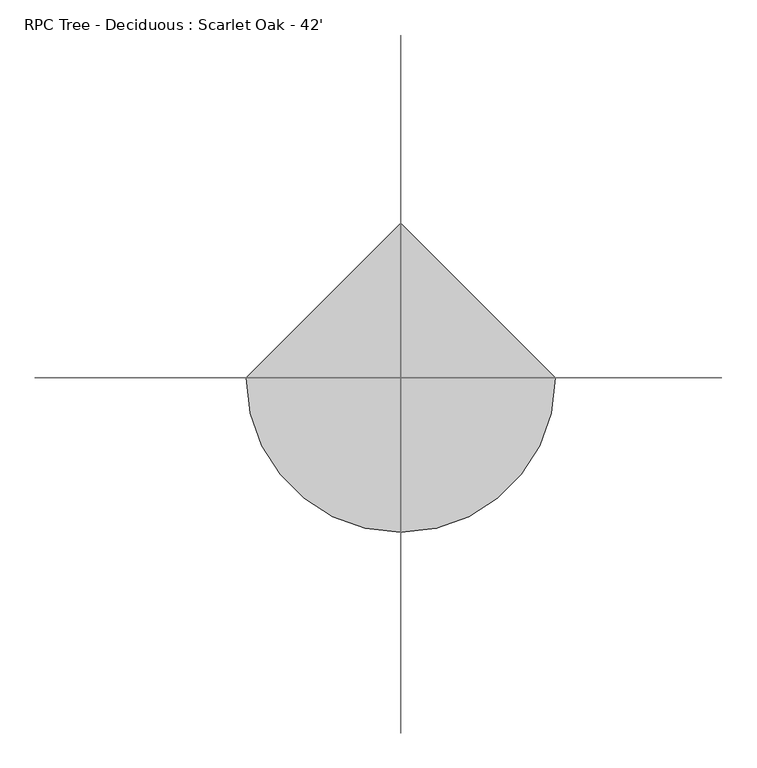
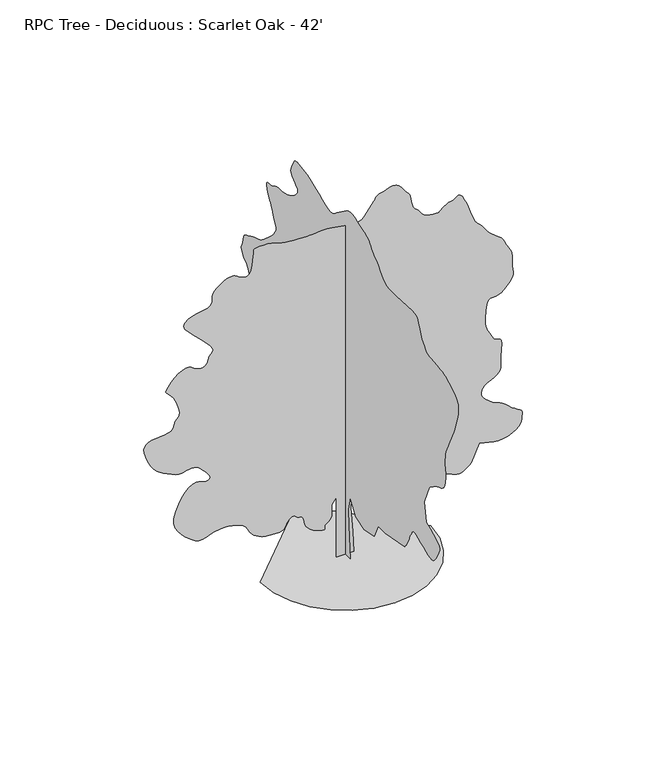
"""IFC4 building model written with IfcOpenShell, lengths in millimetres: geographic element geometry, RPC Tree - Deciduous : Scarlet Oak - 42'."""

from ifc_helpers import new_model, si_unit, origin, place, context, project, spatial, triangles, source, transform, mapped, element, save


def rpc_tree_deciduous_scarlet_oak_42_9b182cbb(model_context):
    return source(origin(), model_context, "Body", "Tessellation", [
        triangles([(0.0176667, 313.3908637, 0.0), (0.0176667, -300.6481277, 0.0), (0.0176667, -201.6098415, 1168.65294), (0.0176667, -181.8016574, 1723.2669067), (0.0176667, -300.6481277, 2238.2675938), (0.0176667, -617.5722605, 1723.2669067), (0.0176667, -1132.5703314, 1564.8060848), (0.0176667, -1726.8001213, 1703.4602669), (0.0176667, -1964.4925896, 2198.6516979), (0.0176667, -2380.4549904, 2198.6516979), (0.0176667, -3529.2988197, 2416.5375263), (0.0176667, -3571.5694954, 2467.5287453), (0.0176667, -3612.8163963, 2518.865728), (0.0176667, -3651.9637161, 2570.8942383), (0.0176667, -3687.9873894, 2623.969487), (0.0176667, -3719.8633507, 2678.4275002), (0.0176667, -3746.5419548, 2734.6266861), (0.0176667, -3766.9988457, 2792.8740028), (0.0176667, -3786.866819, 2852.8877815), (0.0176667, -3811.9324402, 2913.9259163), (0.0176667, -3841.3248322, 2975.8343468), (0.0176667, -3874.1736992, 3038.4340141), (0.0176667, -3909.6343254, 3101.5461502), (0.0176667, -3946.8099632, 3165.016404), (0.0176667, -3984.882058, 3228.6404274), (0.0176667, -4003.0091492, 3249.1996376), (0.0176667, -4028.0747704, 3265.7904854), (0.0176667, -4066.991581, 3274.393158), (0.0176667, -4126.698111, 3271.0392929), (0.0176667, -4214.133181, 3251.7599464), (0.0176667, -4336.2091599, 3212.5358871), (0.0176667, -4499.8648682, 3149.4240417), (0.0176667, -4672.6607162, 3075.1492149), (0.0176667, -4819.8023163, 3008.8625633), (0.0176667, -4944.7714325, 2956.0686928), (0.0176667, -5051.0248306, 2922.3492393), (0.0176667, -5142.0442749, 2913.2343887), (0.0176667, -5221.2603699, 2934.2546173), (0.0176667, -5292.1816223, 2990.9656906), (0.0176667, -5363.7423706, 3080.2954124), (0.0176667, -5437.7099487, 3189.0320892), (0.0176667, -5506.8388687, 3307.4725342), (0.0176667, -5563.8313202, 3425.9129791), (0.0176667, -5601.4168167, 3534.6496559), (0.0176667, -5612.3492889, 3624.0049576), (0.0176667, -5589.3065094, 3684.2236656), (0.0176667, -5533.0052948, 3729.5668282), (0.0176667, -5451.7404877, 3780.0820587), (0.0176667, -5349.7118317, 3834.9496399), (0.0176667, -5231.0155884, 3893.2736961), (0.0176667, -5099.8759186, 3954.2095116), (0.0176667, -4960.4152451, 4016.8603386), (0.0176667, -4816.8068596, 4080.3820427), (0.0176667, -4697.9568466, 4753.8484932), (0.0176667, -4995.0561539, 5447.1064682), (0.0176667, -5004.4270935, 5460.3434509), (0.0176667, -5018.9698105, 5476.4988602), (0.0176667, -5043.9328217, 5498.5690247), (0.0176667, -5084.4629059, 5529.4717896), (0.0176667, -5145.7824188, 5572.1267441), (0.0176667, -5233.1148788, 5629.5290543), (0.0176667, -5351.6064835, 5704.6233078), (0.0176667, -5480.1602646, 5772.6511322), (0.0176667, -5594.1457489, 5817.0984192), (0.0176667, -5693.5885162, 5853.2497009), (0.0176667, -5778.4885666, 5896.340094), (0.0176667, -5848.8209015, 5961.6029709), (0.0176667, -5904.609938, 6064.2717041), (0.0176667, -5945.8312592, 6219.6064087), (0.0176667, -5969.6931747, 6372.1755844), (0.0176667, -5976.5549652, 6470.0056595), (0.0176667, -5971.3064484, 6533.5267822), (0.0176667, -5958.7607025, 6583.1970062), (0.0176667, -5943.8087082, 6639.4476425), (0.0176667, -5931.2885422, 6722.7088394), (0.0176667, -5926.0400253, 6853.4648117), (0.0176667, -5927.8835175, 6997.7129837), (0.0176667, -5935.9737213, 7117.3568436), (0.0176667, -5954.1011032, 7226.6309875), (0.0176667, -5986.0793839, 7339.6950165), (0.0176667, -6035.7496078, 7470.7835266), (0.0176667, -6106.9010788, 7634.1061157), (0.0176667, -6203.3225189, 7843.8473831), (0.0176667, -6294.8797211, 8033.439299), (0.0176667, -6355.9178558, 8147.834642), (0.0176667, -6397.1897552, 8218.5762543), (0.0176667, -6429.4755753, 8277.1819794), (0.0176667, -6463.5019867, 8355.1946594), (0.0176667, -6509.9718246, 8484.1577179), (0.0176667, -6579.6896622, 8695.5634186), (0.0176667, -6654.8094955, 8940.125235), (0.0176667, -6705.3500153, 9150.7373795), (0.0176667, -6723.656456, 9332.2385101), (0.0176667, -6702.0984695, 9489.4934464), (0.0176667, -6633.0980301, 9627.3408463), (0.0176667, -6508.9992096, 9750.6205307), (0.0176667, -6322.1728226, 9864.2211548), (0.0176667, -6140.9019104, 9957.5968506), (0.0176667, -6021.6679092, 10021.8859497), (0.0176667, -5939.1485275, 10064.3101044), (0.0176667, -5868.0487976, 10092.2177032), (0.0176667, -5783.0970062, 10112.8292358), (0.0176667, -5658.9987671, 10133.4396057), (0.0176667, -5470.4567871, 10161.3472046), (0.0176667, -5268.216806, 10183.3400482), (0.0176667, -5111.3717285, 10191.8406921), (0.0176667, -4987.0938492, 10202.3888855), (0.0176667, -4882.5816238, 10230.6290222), (0.0176667, -4784.982058, 10292.127594), (0.0176667, -4681.493898, 10402.5034149), (0.0176667, -4559.2897293, 10577.2962341), (0.0176667, -4452.5756035, 10769.4740387), (0.0176667, -4389.5149178, 10923.9122864), (0.0176667, -4348.2938873, 11044.0165833), (0.0176667, -4307.0469864, 11133.2960175), (0.0176667, -4243.9863007, 11195.2038666), (0.0176667, -4137.2721748, 11233.1992218), (0.0176667, -3965.0652443, 11250.763266), (0.0176667, -3014.2904297, 11191.3378235), (0.0176667, -2839.0363014, 11194.4108917), (0.0176667, -2696.349662, 11194.0004517), (0.0176667, -2575.1186897, 11201.2209412), (0.0176667, -2464.3027794, 11227.1309875), (0.0176667, -2352.7906906, 11282.8694458), (0.0176667, -2229.4985069, 11379.4705261), (0.0176667, -2083.3375156, 11528.0707581), (0.0176667, -1942.4917522, 11678.1569458), (0.0176667, -1836.9835121, 11780.4158203), (0.0176667, -1758.5045815, 11847.7012482), (0.0176667, -1698.7339565, 11892.8147736), (0.0176667, -1649.3606621, 11928.556778), (0.0176667, -1602.0639851, 11967.7555481), (0.0176667, -1548.5328049, 12023.2626251), (0.0176667, -1497.1368141, 12088.8074615), (0.0176667, -1455.0938862, 12149.8444336), (0.0176667, -1412.3621922, 12206.7351471), (0.0176667, -1358.8872585, 12259.7853973), (0.0176667, -1284.6226055, 12309.4044617), (0.0176667, -1179.5189192, 12355.8992981), (0.0176667, -1033.5320452, 12399.6036072), (0.0176667, -869.6434296, 12447.7634583), (0.0176667, -716.8409832, 12501.1206665), (0.0176667, -574.0851983, 12550.3304535), (0.0176667, -440.341763, 12586.0212982), (0.0176667, -314.5660463, 12598.8484222), (0.0176667, -195.7190492, 12579.4414673), (0.0176667, -82.7633712, 12518.4544922), (0.0176667, 511.4674361, 12082.6880676), (0.0176667, 575.7980298, 12024.1335022), (0.0176667, 638.0522604, 11970.7762939), (0.0176667, 705.8469595, 11927.7882202), (0.0176667, 786.8119303, 11900.4189606), (0.0176667, 888.5641497, 11893.8379669), (0.0176667, 1018.7282976, 11913.2460846), (0.0176667, 1184.9289087, 11963.8371826), (0.0176667, 1373.534911, 12038.957016), (0.0176667, 1563.5259304, 12123.4483704), (0.0176667, 1751.4381523, 12209.6791534), (0.0176667, 1933.8071079, 12289.996344), (0.0176667, 2107.1689098, 12356.8213348), (0.0176667, 2268.0542931, 12402.4976166), (0.0176667, 2413.0043118, 12419.4210022), (0.0176667, 2544.8429214, 12428.6634613), (0.0176667, 2667.3156784, 12449.6842712), (0.0176667, 2778.3824455, 12472.4200928), (0.0176667, 2875.9049812, 12486.8599091), (0.0176667, 2957.8610252, 12482.9427063), (0.0176667, 3022.1248352, 12450.606308), (0.0176667, 3066.6488617, 12379.7873749), (0.0176667, 3106.4362587, 12290.8160614), (0.0176667, 3152.1122498, 12208.7582794), (0.0176667, 3195.0232933, 12130.8479187), (0.0176667, 3226.5152664, 12054.318869), (0.0176667, 3237.8831772, 11976.4340881), (0.0176667, 3220.4984825, 11894.3763062), (0.0176667, 3165.7076408, 11805.3794128), (0.0176667, 3081.8572357, 11723.8332275), (0.0176667, 2992.092366, 11659.9534058), (0.0176667, 2909.982843, 11604.7532867), (0.0176667, 2848.9961586, 11549.1938873), (0.0176667, 2822.6759628, 11484.2897095), (0.0176667, 2844.4900383, 11401.0285126), (0.0176667, 2928.0076149, 11290.3713135), (0.0176667, 3043.3244133, 11180.1233917), (0.0176667, 3152.0610901, 11099.7038818), (0.0176667, 3254.9091728, 11042.4550507), (0.0176667, 3352.5598984, 11001.8738068), (0.0176667, 3445.704213, 10971.3035797), (0.0176667, 3535.0595146, 10944.2412781), (0.0176667, 3621.2652992, 10914.0291687), (0.0176667, 3707.3690552, 10890.7561707), (0.0176667, 3795.9049301, 10883.0752441), (0.0176667, 3886.8473442, 10882.333429), (0.0176667, 3980.222168, 10879.8498596), (0.0176667, 4076.0294014, 10866.9715759), (0.0176667, 4174.2690445, 10835.0177124), (0.0176667, 4274.9152267, 10775.3887939), (0.0176667, 4378.9408539, 10722.4152832), (0.0176667, 4481.2000191, 10703.4176056), (0.0176667, 4572.7316414, 10698.9632263), (0.0176667, 4644.5228989, 10689.6684448), (0.0176667, 4687.5362617, 10656.1286316), (0.0176667, 4692.7850693, 10578.9089264), (0.0176667, 4651.2820793, 10438.6546967), (0.0176667, 4589.9369865, 10291.0520782), (0.0176667, 4539.012188, 10191.6093109), (0.0176667, 4494.308812, 10120.561322), (0.0176667, 4451.7053078, 10058.1918732), (0.0176667, 4407.0019318, 9984.7358917), (0.0176667, 4356.0515533, 9880.4538849), (0.0176667, 4294.7320404, 9725.5801987), (0.0176667, 4229.9301819, 9573.2412415), (0.0176667, 4174.1664345, 9477.02444), (0.0176667, 4131.5370598, 9417.880957), (0.0176667, 4106.2412201, 9376.7625366), (0.0176667, 4102.4263367, 9334.6197601), (0.0176667, 4124.265992, 9272.3526306), (0.0176667, 4175.8820274, 9170.9640518), (0.0176667, 4267.7717674, 9036.5728363), (0.0176667, 4396.7095367, 8893.8861969), (0.0176667, 4546.4626053, 8751.5320953), (0.0176667, 4700.6962143, 8618.1908157), (0.0176667, 4843.178215, 8502.5153183), (0.0176667, 4957.5729767, 8413.1858871), (0.0176667, 5027.6233521, 8358.830484), (0.0176667, 5089.8137421, 8324.829071), (0.0176667, 5183.1888565, 8290.4695404), (0.0176667, 5295.279689, 8255.4187729), (0.0176667, 5413.6172333, 8219.3186508), (0.0176667, 5525.7080658, 8181.8354736), (0.0176667, 5619.0831802, 8142.6367035), (0.0176667, 5681.2729889, 8101.3392242), (0.0176667, 5733.3500427, 8067.0308533), (0.0176667, 5799.6622742, 8042.7846588), (0.0176667, 5872.5293381, 8019.2297012), (0.0176667, 5944.3714645, 7986.9950409), (0.0176667, 6007.5606308, 7936.7614792), (0.0176667, 6054.4397461, 7859.1324966), (0.0176667, 6077.431366, 7744.7888947), (0.0176667, 6096.2499847, 7629.9325333), (0.0176667, 6128.5869644, 7548.6938873), (0.0176667, 6163.6888916, 7488.5777893), (0.0176667, 6190.8535126, 7437.1152328), (0.0176667, 6199.277417, 7381.8633728), (0.0176667, 6178.2571884, 7310.3026245), (0.0176667, 6117.0399948, 7209.9889801), (0.0176667, 6041.0492844, 7116.0255295), (0.0176667, 5979.6018723, 7059.8522141), (0.0176667, 5927.8579376, 7023.4183914), (0.0176667, 5880.9526611, 6988.7007431), (0.0176667, 5834.0729645, 6937.699205), (0.0176667, 5782.3290298, 6852.4148758), (0.0176667, 5720.8816177, 6714.7976944), (0.0176667, 5653.9037292, 6576.9502945), (0.0176667, 5592.4557358, 6490.0526917), (0.0176667, 5542.0942749, 6434.6729324), (0.0176667, 5508.3748215, 6391.4034805), (0.0176667, 5496.8278519, 6340.8885406), (0.0176667, 5512.9832611, 6263.6694168), (0.0176667, 5562.4232666, 6140.3897324), (0.0176667, 5628.0954208, 6005.5380798), (0.0176667, 5689.9271118, 5900.8462143), (0.0176667, 5749.0194351, 5817.6361771), (0.0176667, 5806.3450058, 5747.2271027), (0.0176667, 5863.0049194, 5680.9916107), (0.0176667, 5919.9973709, 5610.2499985), (0.0176667, 5978.3728775, 5526.348143), (0.0176667, 6046.1187424, 5443.5985428), (0.0176667, 6124.9511398, 5376.0828964), (0.0176667, 6206.5484848, 5314.8145432), (0.0176667, 6282.6153534, 5250.7556625), (0.0176667, 6344.8057434, 5174.9445923), (0.0176667, 6384.8236496, 5078.3179321), (0.0176667, 6394.3480682, 4951.9151825), (0.0176667, 6402.3615326, 4852.6511833), (0.0176667, 6431.8824051, 4819.9049263), (0.0176667, 6465.5506989, 4818.343103), (0.0176667, 6486.0587494, 4812.6335678), (0.0176667, 6476.0477325, 4767.4183044), (0.0176667, 6418.2611435, 4647.3648766), (0.0176667, 6295.3145782, 4417.1152679), (0.0176667, 6166.7613785, 4158.8557411), (0.0176667, 6089.1579758, 3968.8801277), (0.0176667, 6040.640007, 3832.9270889), (0.0176667, 5999.4186859, 3736.8381866), (0.0176667, 5943.629068, 3666.3782433), (0.0176667, 5851.4579498, 3607.3629501), (0.0176667, 5701.0903839, 3545.5824188), (0.0176667, 5527.4748184, 3495.4511765), (0.0176667, 5374.6748428, 3474.4309479), (0.0176667, 5234.3438736, 3472.8179649), (0.0176667, 5098.1859055, 3480.9087502), (0.0176667, 4957.8549362, 3488.9736649), (0.0176667, 4805.0549606, 3487.3606819), (0.0176667, 4631.4652657, 3466.3404533), (0.0176667, 4458.3362984, 3447.5221252), (0.0176667, 4308.7625793, 3451.5675179), (0.0176667, 4177.2133415, 3467.3900986), (0.0176667, 4058.1328194, 3483.9042068), (0.0176667, 3945.9908272, 3490.0233101), (0.0176667, 3835.2313087, 3474.6614571), (0.0176667, 3720.2984985, 3426.7324059), (0.0176667, 3610.3072472, 3375.7820274), (0.0176667, 3519.3389626, 3349.1034233), (0.0176667, 3449.5190964, 3332.1285873), (0.0176667, 3402.9213593, 3310.3145119), (0.0176667, 3381.6194618, 3269.0679016), (0.0176667, 3387.6874054, 3193.8969086), (0.0176667, 3423.1991913, 3070.1820763), (0.0176667, 3480.4733116, 2938.7610283), (0.0176667, 3549.1923729, 2845.7701927), (0.0176667, 3627.4614326, 2784.8599571), (0.0176667, 3713.3343887, 2749.5789711), (0.0176667, 3804.9171707, 2733.5255905), (0.0176667, 3900.3145454, 2730.2740448), (0.0176667, 3997.6068626, 2733.448851), (0.0176667, 4373.9740059, 2317.4992401), (0.0176667, 4403.4687172, 2270.6632908), (0.0176667, 4431.7603043, 2222.9646034), (0.0176667, 4457.6450615, 2173.5324463), (0.0176667, 4479.868705, 2121.4991398), (0.0176667, 4497.2533997, 2066.004126), (0.0176667, 4508.5698601, 2006.1771091), (0.0176667, 4512.6152527, 1941.1527351), (0.0176667, 4511.9240158, 1873.3554199), (0.0176667, 4507.0847763, 1806.2519577), (0.0176667, 4493.8992439, 1740.5362015), (0.0176667, 4468.2705757, 1676.8969173), (0.0176667, 4425.9996094, 1616.0304291), (0.0176667, 4362.9389236, 1558.6281189), (0.0176667, 4274.9152267, 1505.3836945), (0.0176667, 4190.9622116, 1460.165815), (0.0176667, 4131.9469185, 1424.9973221), (0.0176667, 4081.5854576, 1397.7989822), (0.0176667, 4023.5942299, 1376.4895271), (0.0176667, 3941.7149254, 1358.992194), (0.0176667, 3819.6389465, 1343.2258598), (0.0176667, 3641.0824036, 1327.1137619), (0.0176667, 3437.9721268, 1329.4230686), (0.0176667, 3250.8126205, 1364.996188), (0.0176667, 3076.1221207, 1425.8652924), (0.0176667, 2910.4438614, 1504.0548512), (0.0176667, 2750.3213676, 1591.6024143), (0.0176667, 2592.2472954, 1680.5352127), (0.0176667, 2432.8109516, 1762.8828026), (0.0176667, 2290.6338741, 1837.7823006), (0.0176667, 2180.6808472, 1908.5239128), (0.0176667, 2093.9423916, 1973.376931), (0.0176667, 2021.411063, 2030.6051239), (0.0176667, 1954.0772369, 2078.4780739), (0.0176667, 1882.9309982, 2115.2646366), (0.0176667, 1798.9653385, 2139.2293076), (0.0176667, 1706.624754, 2159.4404285), (0.0176667, 1615.6720207, 2184.5034336), (0.0176667, 1525.0649059, 2211.9936161), (0.0176667, 1433.7664089, 2239.4811825), (0.0176667, 1340.7321167, 2264.5441875), (0.0176667, 1244.9274994, 2284.7553085), (0.0176667, 1145.3130856, 2297.6899841), (0.0176667, 1043.4456116, 2304.4466938), (0.0176667, 941.5755941, 2308.0849892), (0.0176667, 839.7081202, 2309.1244606), (0.0176667, 737.8407188, 2308.0849892), (0.0176667, 635.9732449, 2305.4861652), (0.0176667, 534.1032274, 2301.8480152), (0.0176667, 432.2357898, 2297.6899841), (0.0176667, 234.1596897, 2000.5751255), (0.0176667, 194.5438665, 1544.999445), (287.211575, 0.0006153, 0.0094345), (-307.0182149, 0.0006153, 0.0094345), (-307.0182149, 0.0004871, 2178.8527611), (-465.4815439, 0.0004871, 1960.9695488), (-465.4815439, 0.0005127, 1723.2770805), (-461.8433212, 0.0005127, 1668.1278305), (-461.8433212, 0.0005127, 1613.1500816), (-469.1197666, 0.0005127, 1558.5205673), (-487.308264, 0.0005384, 1504.4107887), (-520.0521955, 0.0005384, 1450.9948631), (-570.9872043, 0.0005384, 1398.4416756), (-643.748933, 0.0005384, 1346.9305756), (-700.7467621, 0.0005384, 1293.4557873), (-716.5132416, 0.0005384, 1239.2870007), (-712.8750189, 0.0005384, 1191.0121857), (-711.6614302, 0.0005384, 1155.206159), (-734.7042824, 0.0005384, 1138.4590708), (-803.8278248, 0.0005384, 1147.3536587), (-940.8638643, 0.0005384, 1188.4698263), (-1097.1892788, 0.0005384, 1252.5136642), (-1214.0141247, 0.0005384, 1324.8708755), (-1297.9209217, 0.0005384, 1404.1613846), (-1355.4973492, 0.0005384, 1488.9925438), (-1393.3235287, 0.0005127, 1577.9815887), (-1417.9820526, 0.0005127, 1669.7434296), (-1436.0578388, 0.0005127, 1762.8929764), (-1440.6767429, 0.0005127, 1788.2427372), (-1447.5485619, 0.0005127, 1812.9011158), (-1458.9240303, 0.0005127, 1836.1770206), (-1477.0588245, 0.0005127, 1857.3687504), (-1504.1983017, 0.0005127, 1875.7903004), (-1542.6030796, 0.0005127, 1890.7476723), (-1594.5186607, 0.0005127, 1901.5471584), (-1646.4342419, 0.0005127, 1919.331102), (-1687.2611103, 0.0005127, 1949.2458458), (-1722.8930923, 0.0004871, 1981.5852962), (-1759.2163113, 0.0004871, 2006.6483013), (-1802.1247387, 0.0004871, 2014.733709), (-1857.5044979, 0.0004871, 1996.138187), (-1931.2494152, 0.0005127, 1941.1604382), (-1996.0996719, 0.0005127, 1864.2407146), (-2032.88638, 0.0005127, 1789.0516994), (-2059.6238468, 0.0005127, 1719.7541851), (-2094.3289959, 0.0005127, 1660.5031506), (-2155.0238377, 0.0005127, 1615.4620045), (-2259.7204994, 0.0005127, 1588.7809296), (-2426.4408463, 0.0005127, 1584.6230438), (-2610.6557648, 0.0005127, 1596.8664825), (-2760.2297745, 0.0005127, 1617.0776035), (-2881.7168358, 0.0005127, 1645.9528759), (-2981.7488113, 0.0005127, 1684.1810658), (-3066.8793709, 0.0005127, 1732.4584969), (-3143.6633469, 0.0005127, 1791.4788769), (-3218.7576004, 0.0005127, 1861.9312626), (-3282.4327835, 0.0005127, 1939.1966045), (-3328.1343544, 0.0004871, 2016.8126518), (-3366.8721062, 0.0004871, 2092.6929039), (-3409.782859, 0.0004871, 2164.7633595), (-3467.9278564, 0.0004871, 2230.9424595), (-3552.4183388, 0.0004871, 2289.1538773), (-3674.3152588, 0.0004871, 2337.3161991), (-3796.8778358, 0.0004871, 2373.9261738), (-3885.797699, 0.0004615, 2399.7981411), (-3956.0271332, 0.0004615, 2416.3148655), (-4022.4419746, 0.0004615, 2424.8611462), (-4099.9171875, 0.0004615, 2426.8249798), (-4203.4053474, 0.0004615, 2423.5911655), (-4347.7817093, 0.0004615, 2416.5452293), (-4506.5217293, 0.0004615, 2391.541087), (-4647.6209656, 0.0004871, 2345.0533722), (-4777.6083801, 0.0004871, 2294.4077717), (-4903.0896744, 0.0004871, 2256.9298267), (-5030.6702591, 0.0004871, 2249.9426079), (-5166.8793869, 0.0004871, 2290.7694763), (-5318.3480484, 0.0004615, 2396.7385895), (-5476.8319794, 0.0004615, 2538.4523232), (-5623.153862, 0.0004615, 2679.118737), (-5747.6625412, 0.0004358, 2825.0057625), (-5840.6277969, 0.0004358, 2982.3118584), (-5892.3717316, 0.0004358, 3157.2843178), (-5893.1908676, 0.0004102, 3356.1698524), (-5833.3561478, 0.0004102, 3585.1904663), (-5733.2221436, 0.0003846, 3816.1824715), (-5621.6434891, 0.0003846, 4014.2744499), (-5501.7694107, 0.0003589, 4175.6259384), (-5376.6973938, 0.0003589, 4296.4217628), (-5249.5266678, 0.0003589, 4372.8729103), (-5123.4052963, 0.0003589, 4401.1900772), (-5001.4313461, 0.0003589, 4377.5072205), (-4886.3965073, 0.0003589, 4337.6686638), (-4784.5469101, 0.0003589, 4320.6679573), (-4704.1526894, 0.0003589, 4327.6064873), (-4653.5607193, 0.0003589, 4359.4824486), (-4641.0920036, 0.0003589, 4417.3457771), (-4675.0419662, 0.0003589, 4502.2458275), (-4763.7313202, 0.0003333, 4615.2072464), (-4867.1683205, 0.0003333, 4728.5014938), (-4946.0004272, 0.0003333, 4815.808374), (-5009.573291, 0.0003333, 4880.2515335), (-5067.2575607, 0.0003333, 4924.9546188), (-5128.4235947, 0.0003333, 4953.0156967), (-5202.3911728, 0.0003076, 4967.5839935), (-5298.5568146, 0.0003076, 4971.7319962), (-5397.1804459, 0.0003333, 4962.437796), (-5478.8545303, 0.0003333, 4941.0077087), (-5553.2313858, 0.0003333, 4917.171373), (-5630.0412323, 0.0003333, 4900.5805252), (-5718.9613861, 0.0003333, 4900.9903839), (-5829.7209045, 0.0003333, 4928.0782654), (-5972.0232651, 0.0003076, 4991.5488098), (-6123.0309082, 0.0003076, 5067.4877792), (-6256.0140701, 0.0003076, 5133.3645721), (-6374.8126328, 0.0003076, 5201.008699), (-6483.1909012, 0.0003076, 5282.1450256), (-6585.0149185, 0.0003076, 5388.5519028), (-6684.0484085, 0.000282, 5532.0576782), (-6784.1312531, 0.000282, 5724.4401215), (-6866.8808533, 0.0002564, 5924.068634), (-6912.5565536, 0.0002564, 6084.5495361), (-6922.9006897, 0.0002564, 6210.3889481), (-6899.6271103, 0.0002307, 6306.0679916), (-6844.4775696, 0.0002307, 6376.118367), (-6759.1938217, 0.0002307, 6425.0206146), (-6645.4641357, 0.0002307, 6457.3064346), (-6511.2008194, 0.0002307, 6475.8430939), (-6369.3338974, 0.0002307, 6486.7755661), (-6229.1564072, 0.0002307, 6499.3980515), (-6100.090448, 0.0002307, 6523.1320679), (-5991.4813797, 0.0002307, 6567.3229752), (-5912.6495636, 0.0002307, 6641.2911346), (-5872.9641953, 0.0002051, 6754.4313217), (-5843.6485428, 0.0002051, 6863.6804672), (-5798.3565399, 0.0002051, 6934.8313568), (-5750.3251694, 0.0002051, 6990.3907562), (-5712.6629333, 0.0002051, 7052.8625244), (-5698.5812347, 0.0001795, 7144.8034241), (-5721.2141556, 0.0001795, 7288.7190582), (-5793.7481003, 0.0001795, 7507.1144485), (-5896.4679932, 0.0001538, 7722.232132), (-5994.7079269, 0.0001538, 7857.6477036), (-6079.0702194, 0.0001538, 7937.9904739), (-6140.2362534, 0.0001282, 7987.8141769), (-6168.8095093, 0.0001282, 8031.7492859), (-6155.4702072, 0.0001282, 8094.4262741), (-6090.8474075, 0.0001282, 8200.3977127), (-5986.6938812, 0.0001282, 8332.6384781), (-5866.2308853, 0.0001025, 8453.101474), (-5737.4468857, 0.0001025, 8554.8481705), (-5608.304187, 0.0001025, 8630.9667801), (-5486.816835, 0.0001025, 8674.4920303), (-5380.8965561, 0.0001025, 8678.5377136), (-5298.5568146, 0.0001025, 8636.1641373), (-5217.8297653, 0.0001025, 8572.9755524), (-5118.386998, 0.0001025, 8523.663446), (-5010.6232269, 0.0001025, 8494.7832321), (-4904.9331665, 0.0001025, 8492.93974), (-4811.7374016, 0.0001025, 8524.713382), (-4741.4053574, 0.0001025, 8596.6584091), (-4704.3320389, 0.0001025, 8715.3802322), (-4670.3564964, 0.0001025, 8828.5721603), (-4616.9995789, 7.69e-05, 8895.677948), (-4566.0747803, 7.69e-05, 8940.9449524), (-4539.3961761, 7.69e-05, 8988.6432037), (-4558.8034218, 7.69e-05, 9063.0206406), (-4646.110302, 7.69e-05, 9188.3484558), (-4823.1820518, 5.13e-05, 9388.8472641), (-5045.2129761, 5.13e-05, 9615.3328583), (-5243.6892334, 2.56e-05, 9806.1281891), (-5404.7584717, 2.56e-05, 9966.78815), (-5514.5197952, 2.56e-05, 10102.8437988), (-5559.1717209, 0.0, 10219.8506104), (-5524.8121902, 0.0, 10323.3384796), (-5397.5897232, 0.0, 10418.8384644), (-5227.9175217, 0.0, 10492.422345), (-5075.9366821, 0.0, 10534.4628021), (-4942.313443, 0.0, 10557.0951416), (-4827.7393318, -2.56e-05, 10572.4569946), (-4732.9050041, -2.56e-05, 10592.6580872), (-4658.527858, -2.56e-05, 10629.8593048), (-4605.2732597, -2.56e-05, 10696.1459564), (-4578.7225548, -2.56e-05, 10774.5690765), (-4574.6774529, -2.56e-05, 10843.2881378), (-4579.2858925, -2.56e-05, 10907.1679596), (-4578.7225548, -2.56e-05, 10971.0477814), (-4559.0850906, -5.13e-05, 11039.7668427), (-4506.5217293, -5.13e-05, 11118.1899628), (-4407.2068611, -5.13e-05, 11211.1552185), (-4285.6427696, -5.13e-05, 11303.1472778), (-4174.4736832, -5.13e-05, 11374.7080261), (-4071.9840088, -7.69e-05, 11424.7619476), (-3976.4072845, -7.69e-05, 11452.3114288), (-3886.0282082, -7.69e-05, 11456.3053711), (-3799.1053162, -7.69e-05, 11435.6694214), (-3713.9488861, -5.13e-05, 11389.4303833), (-3626.1556984, -5.13e-05, 11332.8977875), (-3535.6225616, -5.13e-05, 11288.8353607), (-3446.8053085, -5.13e-05, 11267.2773743), (-3364.2091873, -5.13e-05, 11278.3115845), (-3292.3667702, -5.13e-05, 11331.9501709), (-3235.783596, -7.69e-05, 11438.2808899), (-3198.9404961, -7.69e-05, 11607.3135956), (-3176.9473618, -7.69e-05, 11788.8141449), (-3161.1759407, -0.0001025, 11929.0683746), (-3150.6018768, -0.0001025, 12032.966684), (-3144.2011047, -0.0001025, 12105.3204071), (-3140.8981087, -0.0001025, 12150.9966888), (-3139.6946938, -0.0001025, 12174.8591858), (-3139.5156349, -0.0001025, 12181.7203949), (-3113.477108, -0.0001025, 12185.7666595), (-3042.7354958, -0.0001025, 12194.6765808), (-2938.3767494, -0.0001025, 12203.5609222), (-2811.5129814, -0.0001025, 12207.6060242), (-2673.2045631, -0.0001025, 12201.9470673), (-2534.5452942, -0.0001025, 12181.7203949), (-2406.6342064, -0.0001025, 12142.1123474), (-2289.3460167, -0.0001025, 12098.0499207), (-2171.7120632, -0.0001025, 12066.1227997), (-2048.5351341, -0.0001025, 12043.872995), (-1914.6149654, -0.0001025, 12028.921582), (-1764.7594322, -0.0001025, 12018.8338257), (-1593.7659451, -0.0001025, 12011.1528992), (-1396.4394722, -0.0001025, 12003.4719727), (-1205.9875071, -0.0001025, 12002.3708771), (-1049.1423569, -0.0001025, 12011.6644958), (-911.0079105, -0.0001025, 12024.772998), (-776.6858768, -0.0001025, 12035.1165527), (-631.2776012, -0.0001025, 12036.0897491), (-459.8795603, -0.0001025, 12021.1371735), (-247.5965149, -0.0001025, 11983.6545776), (-33.003293, -0.0001025, 11939.0793915), (140.0111032, -0.0001025, 11908.3556854), (278.3759043, -0.0001025, 11893.2240509), (389.0226934, -0.0001025, 11895.4006622), (478.8797087, -0.0001025, 11916.6761078), (554.8751063, -0.0001025, 11958.7165649), (623.9422932, -0.0001025, 12023.2626251), (921.0572245, -0.0001282, 12399.6036072), (965.640041, -0.0001282, 12457.6465759), (1001.2131603, -0.0001282, 12512.2327789), (1033.3195581, -0.0001282, 12562.2867004), (1067.507515, -0.0001282, 12606.8107269), (1109.3175356, -0.0001282, 12644.7549225), (1164.2952845, -0.0001282, 12675.0693512), (1237.9812664, -0.0001282, 12696.729657), (1328.2991547, -0.0001538, 12721.5641876), (1426.9329597, -0.0001538, 12754.7203033), (1530.070269, -0.0001538, 12785.0858917), (1633.9040474, -0.0001538, 12801.6), (1734.6167953, -0.0001538, 12793.1760956), (1828.3987164, -0.0001538, 12748.7032288), (1911.4427753, -0.0001282, 12657.1216095), (1985.1850765, -0.0001282, 12552.6605438), (2052.6930199, -0.0001282, 12471.3957367), (2112.5788994, -0.0001282, 12405.0323456), (2163.4550091, -0.0001282, 12345.2743652), (2203.9362591, -0.0001282, 12283.7757935), (2232.6374142, -0.0001025, 12212.2138824), (2248.1709137, -0.0001025, 12122.2961151), (2258.9703999, -0.0001025, 12029.1006409), (2273.9277718, -0.0001025, 11951.4972382), (2292.3491764, -0.0001025, 11886.8744385), (2313.5410515, -7.69e-05, 11832.6463531), (2336.8143402, -7.69e-05, 11786.2026764), (2361.4727188, -7.69e-05, 11744.9819366), (2386.8250957, -7.69e-05, 11706.3459229), (2412.4640831, -7.69e-05, 11688.9621002), (2439.1453033, -7.69e-05, 11669.1447052), (2467.9025597, -7.69e-05, 11644.4892334), (2499.7811371, -7.69e-05, 11612.5621124), (2535.8152748, -7.69e-05, 11570.9309326), (2577.0389214, -7.69e-05, 11517.164447), (2624.5072449, -7.69e-05, 11448.8546631), (2694.8648689, -5.13e-05, 11383.9249054), (2794.3076363, -5.13e-05, 11339.4776184), (2908.2931206, -5.13e-05, 11311.6223419), (3022.2786049, -5.13e-05, 11296.6186066), (3121.7213722, -5.13e-05, 11290.601532), (3192.0789963, -5.13e-05, 11289.8073944), (3218.7576004, -5.13e-05, 11290.3968933), (3232.429731, -5.13e-05, 11304.6576508), (3270.0408073, -5.13e-05, 11341.4240112), (3326.3420219, -5.13e-05, 11391.7337311), (3396.1621788, -7.69e-05, 11446.5245728), (3474.2774689, -7.69e-05, 11496.8354553), (3555.5419853, -7.69e-05, 11533.6273956), (3634.7072113, -7.69e-05, 11547.8881531), (3705.6790421, -7.69e-05, 11565.2731384), (3768.3301598, -7.69e-05, 11604.4707458), (3826.500737, -7.69e-05, 11646.1019257), (3883.9542068, -7.69e-05, 11670.7829773), (3944.5313232, -7.69e-05, 11659.0569489), (4012.0469696, -7.69e-05, 11591.5413025), (4090.2904495, -7.69e-05, 11448.8546631), (4163.9763588, -5.13e-05, 11281.2055939), (4218.94655, -5.13e-05, 11145.7894409), (4260.756498, -5.13e-05, 11033.5707092), (4294.9366791, -2.56e-05, 10935.5871552), (4327.0431496, -2.56e-05, 10842.7765411), (4362.631675, -2.56e-05, 10746.1754608), (4407.2068611, -2.56e-05, 10636.7216766), (4453.011042, 0.0, 10540.6833527), (4492.2095215, 0.0, 10479.6452179), (4530.3839355, 0.0, 10437.682663), (4573.0644699, 0.0, 10398.8164307), (4625.7813103, 0.0, 10347.1230743), (4694.0908035, 0.0, 10266.6779846), (4783.5481339, 0.0, 10141.5298096), (4893.6675751, 2.56e-05, 10002.2487762), (5014.5404297, 2.56e-05, 9885.8303009), (5137.4869949, 2.56e-05, 9786.0294159), (5253.8537292, 5.13e-05, 9696.6488251), (5354.9603485, 5.13e-05, 9611.4156555), (5432.1794724, 5.13e-05, 9524.0831955), (5476.8319794, 5.13e-05, 9428.4553116), (5511.8827469, 5.13e-05, 9334.6709198), (5560.7844131, 7.69e-05, 9250.5900055), (5615.6008347, 7.69e-05, 9166.5090912), (5668.3179657, 7.69e-05, 9072.724118), (5710.9985001, 7.69e-05, 8959.5583511), (5735.6545532, 0.0001025, 8817.2554092), (5734.3232391, 0.0001025, 8636.1641373), (5731.6094513, 0.0001025, 8462.1137146), (5746.5614456, 0.0001282, 8335.1732071), (5762.8964951, 0.0001282, 8237.0100128), (5764.3557083, 0.0001282, 8149.2171158), (5734.6046173, 0.0001282, 8053.4863312), (5657.4110733, 0.0001538, 7931.3850632), (5516.4400269, 0.0001538, 7764.6057083), (5349.148494, 0.0001538, 7624.5816971), (5204.0294449, 0.0001538, 7568.3828018), (5081.4159988, 0.0001538, 7556.195755), (4981.691272, 0.0001538, 7548.1817093), (4905.163385, 0.0001795, 7504.4518204), (4852.2160355, 0.0001795, 7385.2172379), (4823.156472, 0.0001795, 7150.5896988), (4812.3007393, 0.0002051, 6890.9474075), (4813.9393021, 0.0002051, 6708.2178635), (4828.3538292, 0.0002307, 6579.9198807), (4855.9797592, 0.0002307, 6483.4728607), (4897.0981796, 0.0002307, 6396.396199), (4952.0686615, 0.0002307, 6296.1342957), (5021.2481598, 0.0002564, 6160.206546), (5100.1828766, 0.0002564, 6041.9969009), (5179.8344101, 0.0002564, 5988.229834), (5253.5717697, 0.0002564, 5966.3393097), (5314.840123, 0.0002564, 5943.7575485), (5357.0602203, 0.0002564, 5887.9167709), (5373.6254883, 0.000282, 5766.2247803), (5357.9816757, 0.000282, 5546.1649567), (5336.7312286, 0.0003076, 5303.5495331), (5333.4796829, 0.0003076, 5126.0935043), (5337.1916656, 0.0003076, 4998.8710373), (5336.7312286, 0.0003333, 4907.0068771), (5321.0106766, 0.0003333, 4835.574028), (5278.9702194, 0.0003333, 4769.6713646), (5199.5233246, 0.0003333, 4694.423632), (5103.537323, 0.0003333, 4623.8610786), (5018.6366913, 0.0003333, 4576.1622459), (4943.7988174, 0.0003333, 4542.6733017), (4877.9726028, 0.0003589, 4514.7145432), (4820.109565, 0.0003589, 4483.6580086), (4769.1847664, 0.0003589, 4440.7981247), (4724.1232727, 0.0003589, 4377.5072205), (4688.3301086, 0.0003589, 4304.2308792), (4668.1034363, 0.0003589, 4235.1022499), (4666.951181, 0.0003589, 4167.0232658), (4688.3301086, 0.0003846, 4096.8447006), (4735.6702423, 0.0003846, 4021.4946487), (4812.4797981, 0.0003846, 3937.7977226), (4922.2152512, 0.0003846, 3842.7075966), (5038.5046646, 0.0003846, 3759.3690788), (5137.1538757, 0.0003846, 3704.7831665), (5224.6915558, 0.0004102, 3666.5061424), (5307.748114, 0.0004102, 3632.0442924), (5392.8533844, 0.0004102, 3588.9030304), (5486.6377762, 0.0004102, 3524.6133499), (5595.6561218, 0.0004102, 3426.7324059), (5711.4083588, 0.0004102, 3325.6252052), (5818.1221939, 0.0004102, 3253.27061), (5911.6763672, 0.0004358, 3199.6064438), (5987.8972961, 0.0004358, 3154.6213989), (6042.6369781, 0.0004358, 3108.254171), (6071.7474106, 0.0004358, 3050.4420021), (6071.0561737, 0.0004358, 2971.148877), (6059.6888443, 0.0004358, 2881.1282089), (6052.801474, 0.0004615, 2796.6374359), (6040.3836273, 0.0004615, 2715.961837), (6012.3737091, 0.0004615, 2637.3855286), (5958.7351227, 0.0004615, 2559.1269333), (5869.4056915, 0.0004615, 2479.4908058), (5734.3232391, 0.0004615, 2396.7385895), (5573.023201, 0.0004871, 2329.7503819), (5411.7481613, 0.0004871, 2294.9863701), (5250.4481232, 0.0004871, 2287.0749344), (5089.148085, 0.0004871, 2300.6446003), (4927.8736267, 0.0004871, 2330.3265095), (4766.5732979, 0.0004871, 2370.7513676), (4605.2732597, 0.0004615, 2416.5452293), (4327.9648956, 0.0005127, 1802.5088722), (4260.0141014, 0.0005127, 1743.6034561), (4191.6790283, 0.0005127, 1687.8192158), (4122.6785889, 0.0005127, 1638.2719494), (4052.6282135, 0.0005127, 1598.0774551), (3981.1950737, 0.0005127, 1570.3595249), (3908.0213425, 0.0005127, 1558.2338116), (3832.7733192, 0.0005127, 1564.816404), (3771.4538063, 0.0005127, 1579.7711597), (3732.639315, 0.0005127, 1592.3039703), (3704.9366455, 0.0005127, 1604.8367809), (3676.8755676, 0.0005127, 1619.7915367), (3637.0114311, 0.0005127, 1639.6007927), (3573.9507454, 0.0005127, 1666.6838779), (3476.2488602, 0.0005127, 1703.4704407), (3348.9752335, 0.0005127, 1756.8865116), (3209.9244186, 0.0005127, 1827.6281239), (3066.7000214, 0.0005127, 1908.7645958), (2926.957679, 0.0004871, 1993.3652458), (2798.2759987, 0.0004871, 2074.5018631), (2688.335907, 0.0004871, 2145.2434753), (2604.716011, 0.0004871, 2198.6620171), (2533.9101585, 0.0004871, 2245.7258595), (2457.9147972, 0.0004871, 2301.1054733), (2377.5848167, 0.0004871, 2363.4185303), (2293.7932743, 0.0004615, 2431.2722374), (2207.4004372, 0.0004615, 2503.2838303), (2119.2767464, 0.0004615, 2578.0629868), (2030.2877014, 0.0004615, 2654.2324654), (2010.4784454, 0.0004358, 2951.3576431), (1614.3253006, 0.0004358, 2990.9656906), (901.2479685, 0.0004358, 2931.5408295), (425.8657207, 0.0004615, 2674.049279), (227.7880946, 0.0004871, 2198.6620171), (188.1730163, 0.0005127, 1644.0454342), (247.5954975, 0.000564, 732.8941458), (-2924.8072289, 0.0, 0.0229709), (-2847.485495, -670.1739916, 0.0229709), (-2627.2724831, -1285.6237072, 0.0229709), (-2281.8083954, -1828.7110519, 0.0229709), (-1828.7110519, -2281.8083954, 0.0229709), (-1285.6237072, -2627.2724831, 0.0229709), (-670.1739916, -2847.485495, 0.0229709), (0.0001278, -2924.8072289, 0.0229709), (670.1739916, -2847.485495, 0.0229709), (1285.6237072, -2627.2724831, 0.0229709), (1828.7110519, -2281.8083954, 0.0229709), (2281.8083954, -1828.7110519, 0.0229709), (2627.2724831, -1285.6237072, 0.0229709), (2847.485495, -670.1739916, 0.0229709), (2924.8072289, 0.0002564, 0.0229709), (-0.0003835, 2924.8072289, 0.0229709)], [[1, 2, 3], [368, 1, 3], [368, 3, 4], [367, 368, 4], [367, 4, 5], [277, 278, 279], [366, 367, 5], [276, 277, 279], [276, 279, 280], [7, 8, 9], [6, 7, 9], [5, 6, 9], [315, 316, 317], [201, 202, 203], [200, 201, 203], [200, 203, 204], [199, 200, 204], [199, 204, 205], [198, 199, 205], [198, 205, 206], [198, 206, 207], [197, 198, 207], [197, 207, 208], [275, 276, 280], [196, 197, 208], [195, 196, 208], [194, 195, 208], [194, 208, 209], [193, 194, 209], [192, 193, 209], [192, 209, 210], [191, 192, 210], [191, 210, 211], [191, 211, 212], [190, 191, 212], [190, 212, 213], [190, 213, 214], [189, 190, 214], [189, 214, 215], [188, 189, 215], [187, 188, 215], [186, 187, 215], [10, 11, 12], [314, 315, 317], [10, 12, 13], [10, 13, 14], [10, 14, 15], [10, 15, 16], [10, 16, 17], [10, 17, 18], [10, 18, 19], [10, 19, 20], [10, 20, 21], [10, 21, 22], [185, 186, 215], [185, 215, 216], [275, 280, 281], [10, 22, 23], [167, 168, 169], [166, 167, 169], [165, 166, 169], [165, 169, 170], [164, 165, 170], [164, 170, 171], [163, 164, 171], [163, 171, 172], [163, 172, 173], [163, 173, 174], [163, 174, 175], [163, 175, 176], [163, 176, 177], [163, 177, 178], [163, 178, 179], [163, 179, 180], [162, 163, 180], [161, 162, 180], [160, 161, 180], [159, 160, 180], [159, 180, 181], [158, 159, 181], [157, 158, 181], [156, 157, 181], [156, 181, 182], [155, 156, 182], [154, 155, 182], [154, 182, 183], [9, 10, 23], [9, 23, 24], [9, 24, 25], [45, 46, 47], [44, 45, 47], [44, 47, 48], [43, 44, 48], [43, 48, 49], [42, 43, 49], [42, 49, 50], [41, 42, 50], [40, 41, 50], [40, 50, 51], [39, 40, 51], [38, 39, 51], [37, 38, 51], [36, 37, 51], [35, 36, 51], [34, 35, 51], [33, 34, 51], [33, 51, 52], [32, 33, 52], [32, 52, 53], [31, 32, 53], [30, 31, 53], [29, 30, 53], [28, 29, 53], [28, 53, 54], [27, 28, 54], [26, 27, 54], [5, 9, 25], [5, 25, 26], [5, 26, 54], [5, 54, 55], [366, 5, 55], [365, 366, 55], [364, 365, 55], [363, 364, 55], [362, 363, 55], [361, 362, 55], [361, 55, 56], [153, 154, 183], [153, 183, 184], [313, 314, 317], [360, 361, 56], [184, 185, 216], [153, 184, 216], [152, 153, 216], [152, 216, 217], [243, 244, 245], [242, 243, 245], [242, 245, 246], [241, 242, 246], [241, 246, 247], [241, 247, 248], [240, 241, 248], [240, 248, 249], [240, 249, 250], [239, 240, 250], [239, 250, 251], [238, 239, 251], [237, 238, 251], [236, 237, 251], [235, 236, 251], [234, 235, 251], [233, 234, 251], [232, 233, 251], [231, 232, 251], [230, 231, 251], [229, 230, 251], [228, 229, 251], [228, 251, 252], [227, 228, 252], [226, 227, 252], [226, 252, 253], [226, 253, 254], [226, 254, 255], [226, 255, 256], [226, 256, 257], [225, 226, 257], [224, 225, 257], [223, 224, 257], [222, 223, 257], [222, 257, 258], [221, 222, 258], [220, 221, 258], [115, 116, 117], [114, 115, 117], [114, 117, 118], [113, 114, 118], [113, 118, 119], [112, 113, 119], [111, 112, 119], [110, 111, 119], [152, 217, 218], [313, 317, 318], [313, 318, 319], [313, 319, 320], [313, 320, 321], [313, 321, 322], [313, 322, 323], [313, 323, 324], [313, 324, 325], [313, 325, 326], [313, 326, 327], [313, 327, 328], [313, 328, 329], [313, 329, 330], [313, 330, 331], [313, 331, 332], [313, 332, 333], [313, 333, 334], [313, 334, 335], [313, 335, 336], [313, 336, 337], [313, 337, 338], [313, 338, 339], [313, 339, 340], [313, 340, 341], [312, 313, 341], [312, 341, 342], [312, 342, 343], [311, 312, 343], [311, 343, 344], [311, 344, 345], [310, 311, 345], [310, 345, 346], [310, 346, 347], [310, 347, 348], [309, 310, 348], [309, 348, 349], [309, 349, 350], [308, 309, 350], [308, 350, 351], [307, 308, 351], [307, 351, 352], [307, 352, 353], [307, 353, 354], [307, 354, 355], [307, 355, 356], [307, 356, 357], [307, 357, 358], [306, 307, 358], [306, 358, 359], [306, 359, 360], [306, 360, 56], [305, 306, 56], [305, 56, 57], [304, 305, 57], [303, 304, 57], [302, 303, 57], [301, 302, 57], [301, 57, 58], [301, 58, 59], [110, 119, 120], [109, 110, 120], [109, 120, 121], [301, 59, 60], [300, 301, 60], [300, 60, 61], [151, 152, 218], [109, 121, 122], [300, 61, 62], [145, 146, 147], [144, 145, 147], [143, 144, 147], [143, 147, 148], [142, 143, 148], [141, 142, 148], [140, 141, 148], [140, 148, 149], [139, 140, 149], [138, 139, 149], [137, 138, 149], [136, 137, 149], [135, 136, 149], [134, 135, 149], [133, 134, 149], [132, 133, 149], [132, 149, 150], [131, 132, 150], [130, 131, 150], [129, 130, 150], [128, 129, 150], [127, 128, 150], [126, 127, 150], [126, 150, 151], [126, 151, 218], [125, 126, 218], [124, 125, 218], [123, 124, 218], [123, 218, 219], [122, 123, 219], [109, 122, 219], [108, 109, 219], [108, 219, 220], [108, 220, 258], [108, 258, 259], [108, 259, 260], [108, 260, 261], [108, 261, 262], [107, 108, 262], [107, 262, 263], [107, 263, 264], [106, 107, 264], [106, 264, 265], [106, 265, 266], [106, 266, 267], [106, 267, 268], [105, 106, 268], [104, 105, 268], [103, 104, 268], [102, 103, 268], [101, 102, 268], [100, 101, 268], [99, 100, 268], [98, 99, 268], [97, 98, 268], [96, 97, 268], [95, 96, 268], [94, 95, 268], [93, 94, 268], [92, 93, 268], [91, 92, 268], [90, 91, 268], [89, 90, 268], [88, 89, 268], [87, 88, 268], [86, 87, 268], [85, 86, 268], [84, 85, 268], [83, 84, 268], [82, 83, 268], [81, 82, 268], [80, 81, 268], [79, 80, 268], [78, 79, 268], [77, 78, 268], [76, 77, 268], [75, 76, 268], [74, 75, 268], [73, 74, 268], [72, 73, 268], [71, 72, 268], [70, 71, 268], [69, 70, 268], [68, 69, 268], [67, 68, 268], [66, 67, 268], [65, 66, 268], [64, 65, 268], [63, 64, 268], [62, 63, 268], [300, 62, 268], [299, 300, 268], [298, 299, 268], [297, 298, 268], [296, 297, 268], [295, 296, 268], [294, 295, 268], [293, 294, 268], [292, 293, 268], [291, 292, 268], [290, 291, 268], [289, 290, 268], [288, 289, 268], [287, 288, 268], [286, 287, 268], [285, 286, 268], [284, 285, 268], [283, 284, 268], [282, 283, 268], [281, 282, 268], [275, 281, 268], [275, 268, 269], [274, 275, 269], [274, 269, 270], [274, 270, 271], [273, 274, 271], [272, 273, 271], [802, 369, 370], [802, 370, 371], [801, 802, 371], [800, 801, 371], [575, 576, 577], [799, 800, 371], [574, 575, 577], [383, 384, 385], [383, 385, 386], [382, 383, 386], [382, 386, 387], [381, 382, 387], [381, 387, 388], [794, 795, 796], [510, 511, 512], [574, 577, 578], [573, 574, 578], [572, 573, 578], [572, 578, 579], [571, 572, 579], [571, 579, 580], [570, 571, 580], [570, 580, 581], [570, 581, 582], [569, 570, 582], [569, 582, 583], [569, 583, 584], [568, 569, 584], [568, 584, 585], [509, 510, 512], [509, 512, 513], [508, 509, 513], [508, 513, 514], [508, 514, 515], [507, 508, 515], [507, 515, 516], [507, 516, 517], [507, 517, 518], [507, 518, 519], [507, 519, 520], [507, 520, 521], [507, 521, 522], [506, 507, 522], [506, 522, 523], [505, 506, 523], [505, 523, 524], [504, 505, 524], [568, 585, 586], [504, 524, 525], [538, 539, 540], [538, 540, 541], [537, 538, 541], [537, 541, 542], [536, 537, 542], [536, 542, 543], [536, 543, 544], [535, 536, 544], [535, 544, 545], [535, 545, 546], [534, 535, 546], [534, 546, 547], [533, 534, 547], [533, 547, 548], [381, 388, 389], [380, 381, 389], [380, 389, 390], [380, 390, 391], [380, 391, 392], [380, 392, 393], [379, 380, 393], [378, 379, 393], [377, 378, 393], [376, 377, 393], [375, 376, 393], [374, 375, 393], [373, 374, 393], [372, 373, 393], [372, 393, 394], [372, 394, 395], [372, 395, 396], [372, 396, 397], [372, 397, 398], [371, 372, 398], [371, 398, 399], [532, 533, 548], [371, 399, 400], [567, 568, 586], [567, 586, 587], [657, 658, 659], [657, 659, 660], [656, 657, 660], [656, 660, 661], [655, 656, 661], [655, 661, 662], [654, 655, 662], [654, 662, 663], [653, 654, 663], [652, 653, 663], [651, 652, 663], [650, 651, 663], [649, 650, 663], [649, 663, 664], [648, 649, 664], [647, 648, 664], [647, 664, 665], [647, 665, 666], [647, 666, 667], [647, 667, 668], [647, 668, 669], [793, 794, 796], [713, 714, 715], [713, 715, 716], [712, 713, 716], [712, 716, 717], [711, 712, 717], [646, 647, 669], [711, 717, 718], [567, 587, 588], [645, 646, 669], [645, 669, 670], [750, 751, 752], [749, 750, 752], [748, 749, 752], [748, 752, 753], [747, 748, 753], [747, 753, 754], [747, 754, 755], [747, 755, 756], [747, 756, 757], [747, 757, 758], [747, 758, 759], [747, 759, 760], [746, 747, 760], [746, 760, 761], [746, 761, 762], [745, 746, 762], [745, 762, 763], [745, 763, 764], [744, 745, 764], [743, 744, 764], [743, 764, 765], [742, 743, 765], [741, 742, 765], [741, 765, 766], [740, 741, 766], [739, 740, 766], [738, 739, 766], [737, 738, 766], [736, 737, 766], [735, 736, 766], [644, 645, 670], [567, 588, 589], [792, 793, 796], [371, 400, 401], [371, 401, 402], [371, 402, 403], [371, 403, 404], [371, 404, 405], [799, 371, 405], [799, 405, 406], [766, 767, 768], [488, 489, 490], [488, 490, 491], [487, 488, 491], [487, 491, 492], [486, 487, 492], [486, 492, 493], [485, 486, 493], [485, 493, 494], [485, 494, 495], [484, 485, 495], [483, 484, 495], [483, 495, 496], [482, 483, 496], [481, 482, 496], [480, 481, 496], [479, 480, 496], [479, 496, 497], [478, 479, 497], [477, 478, 497], [476, 477, 497], [475, 476, 497], [474, 475, 497], [473, 474, 497], [472, 473, 497], [471, 472, 497], [471, 497, 498], [470, 471, 498], [469, 470, 498], [469, 498, 499], [468, 469, 499], [468, 499, 500], [468, 500, 501], [468, 501, 502], [468, 502, 503], [467, 468, 503], [466, 467, 503], [466, 503, 504], [466, 504, 525], [465, 466, 525], [465, 525, 526], [464, 465, 526], [463, 464, 526], [735, 766, 768], [735, 768, 769], [735, 769, 770], [735, 770, 771], [735, 771, 772], [735, 772, 773], [735, 773, 774], [735, 774, 775], [735, 775, 776], [735, 776, 777], [735, 777, 778], [735, 778, 779], [735, 779, 780], [735, 780, 781], [735, 781, 782], [735, 782, 783], [735, 783, 784], [735, 784, 785], [735, 785, 786], [735, 786, 787], [735, 787, 788], [735, 788, 789], [735, 789, 790], [735, 790, 791], [735, 791, 792], [735, 792, 796], [734, 735, 796], [733, 734, 796], [732, 733, 796], [731, 732, 796], [731, 796, 797], [730, 731, 797], [567, 589, 590], [455, 456, 457], [454, 455, 457], [453, 454, 457], [453, 457, 458], [452, 453, 458], [451, 452, 458], [451, 458, 459], [450, 451, 459], [449, 450, 459], [448, 449, 459], [447, 448, 459], [446, 447, 459], [445, 446, 459], [444, 445, 459], [443, 444, 459], [442, 443, 459], [441, 442, 459], [440, 441, 459], [439, 440, 459], [438, 439, 459], [437, 438, 459], [437, 459, 460], [436, 437, 460], [435, 436, 460], [434, 435, 460], [434, 460, 461], [433, 434, 461], [432, 433, 461], [431, 432, 461], [430, 431, 461], [429, 430, 461], [428, 429, 461], [428, 461, 462], [427, 428, 462], [411, 412, 413], [411, 413, 414], [410, 411, 414], [410, 414, 415], [409, 410, 415], [409, 415, 416], [409, 416, 417], [408, 409, 417], [408, 417, 418], [408, 418, 419], [408, 419, 420], [408, 420, 421], [408, 421, 422], [408, 422, 423], [408, 423, 424], [408, 424, 425], [408, 425, 426], [407, 408, 426], [407, 426, 427], [407, 427, 462], [406, 407, 462], [799, 406, 462], [799, 462, 463], [799, 463, 526], [798, 799, 526], [798, 526, 527], [798, 527, 528], [798, 528, 529], [798, 529, 530], [798, 530, 531], [797, 798, 531], [730, 797, 531], [729, 730, 531], [728, 729, 531], [728, 531, 532], [728, 532, 548], [728, 548, 549], [728, 549, 550], [727, 728, 550], [726, 727, 550], [725, 726, 550], [724, 725, 550], [723, 724, 550], [722, 723, 550], [721, 722, 550], [720, 721, 550], [719, 720, 550], [718, 719, 550], [711, 718, 550], [710, 711, 550], [709, 710, 550], [708, 709, 550], [707, 708, 550], [706, 707, 550], [705, 706, 550], [704, 705, 550], [703, 704, 550], [702, 703, 550], [701, 702, 550], [701, 550, 551], [701, 551, 552], [701, 552, 553], [701, 553, 554], [701, 554, 555], [701, 555, 556], [701, 556, 557], [701, 557, 558], [701, 558, 559], [700, 701, 559], [699, 700, 559], [698, 699, 559], [697, 698, 559], [696, 697, 559], [617, 618, 619], [616, 617, 619], [615, 616, 619], [615, 619, 620], [614, 615, 620], [613, 614, 620], [613, 620, 621], [612, 613, 621], [612, 621, 622], [611, 612, 622], [610, 611, 622], [609, 610, 622], [608, 609, 622], [607, 608, 622], [606, 607, 622], [605, 606, 622], [604, 605, 622], [604, 622, 623], [604, 623, 624], [604, 624, 625], [604, 625, 626], [604, 626, 627], [604, 627, 628], [604, 628, 629], [604, 629, 630], [604, 630, 631], [604, 631, 632], [603, 604, 632], [603, 632, 633], [602, 603, 633], [602, 633, 634], [602, 634, 635], [602, 635, 636], [602, 636, 637], [602, 637, 638], [602, 638, 639], [602, 639, 640], [602, 640, 641], [601, 602, 641], [643, 644, 670], [643, 670, 671], [567, 590, 591], [566, 567, 591], [692, 693, 694], [692, 694, 695], [691, 692, 695], [691, 695, 696], [690, 691, 696], [680, 681, 682], [689, 690, 696], [679, 680, 682], [679, 682, 683], [678, 679, 683], [559, 560, 561], [559, 561, 562], [559, 562, 563], [566, 591, 592], [642, 643, 671], [642, 671, 672], [642, 672, 673], [642, 673, 674], [642, 674, 675], [642, 675, 676], [600, 601, 641], [688, 689, 696], [687, 688, 696], [686, 687, 696], [685, 686, 696], [684, 685, 696], [683, 684, 696], [678, 683, 696], [677, 678, 696], [676, 677, 696], [642, 676, 696], [641, 642, 696], [600, 641, 696], [599, 600, 696], [598, 599, 696], [597, 598, 696], [596, 597, 696], [595, 596, 696], [594, 595, 696], [593, 594, 696], [592, 593, 696], [566, 592, 696], [565, 566, 696], [564, 565, 696], [564, 696, 559], [564, 559, 563], [817, 818, 803], [816, 817, 803], [816, 803, 804], [815, 816, 804], [815, 804, 805], [815, 805, 806], [814, 815, 806], [813, 814, 806], [813, 806, 807], [813, 807, 808], [813, 808, 809], [813, 809, 810], [813, 810, 811], [813, 811, 812]], closed=False),
    ])


if __name__ == "__main__":
    model = new_model("IFC4")
    model_context = context("Model", 3, world=origin())
    ifc_project = project(units=[si_unit("LENGTHUNIT", "METRE", prefix="MILLI")], contexts=[model_context])
    site = spatial("IfcSite", under=ifc_project)
    building = spatial("IfcBuilding", under=site)
    placement = place(None, origin())
    rpc_tree_deciduous_scarlet_oak_42_shape = rpc_tree_deciduous_scarlet_oak_42_9b182cbb(model_context)
    element("IfcGeographicElement", 1, ObjectType="RPC Tree - Deciduous : Scarlet Oak - 42'", at=placement, inside=building, context=model_context, shape_type="MappedRepresentation", body=[
        mapped(rpc_tree_deciduous_scarlet_oak_42_shape, transform((0.0, 0.0, 0.0), x_axis=(1.0, 0.0, 0.0), y_axis=(0.0, 1.0, 0.0), z_axis=(0.0, 0.0, 1.0))),
    ])
    save(model, "model.ifc")

# Revit data of these elements
# Type "RPC Tree - Deciduous : Scarlet Oak - 42'"
#   built-in parameter 1005198 = "{2, 15},{39, RPC-16-G0FB-J5PX-0LX6-U000-ST1L-LVER-AU},{1, 0},{1, 0},{2, 13},{1, 8},{5, Color},{1, 0},{1, 0},{3, 0.8},{3, 0.8},{3, 0.8},{1, 8},{7, BBoxMin},{1, 0},{1, 0},{1, 0},{1, 0},{1, 0},{1, 8},{7, BBoxMax},{1, 0},{1, 0},{1, 0},{1, 0},{1, 0},{2, 11},{9, RPCTypeId},{1, 0},{1, 0},{39, RPC-16-G0FB-J5PX-0LX6-U000-ST1L-LVER-AU},{1, 6},{14, RPCPlantHeight},{1, 0},{1, 0},{2, 42},{2, 11},{7, keyword},{1, 0},{1, 0},{34, :RPCs:Trees [General]:Geometry:RPC},{2, 11},{8, category},{1, 0},{1, 0},{15, Trees [General]},{2, 11},{12, LocalizedUID},{1, 0},{1, 0},{11, Scarlet_Oak},{2, 14},{6, Height},{1, 0},{1, 0},{2, 42},{1, 2},{16, Cast Reflections},{1, 0},{1, 0},{1, 0},{1, 2},{12, Cast Shadows},{1, 0},{1, 0},{1, 1},{1, 2},{9, Lock View},{1, 0},{1, 0},{1, 0},{1, 4},{5, ViewC},{1, 0},{1, 0},{1, 0},{21, assetlibrary_base.fbx},{1, 5},"
#   built-in parameter 1005195 = "RPC-16-G0FB-J5PX-0LX6-U000-ST1L-LVER-AU"
#   Type Comments = "Scarlet Oak"
#   Assembly Code = "G2050500"
#   Height = 42' - 0"
#   Default Elevation = 0
